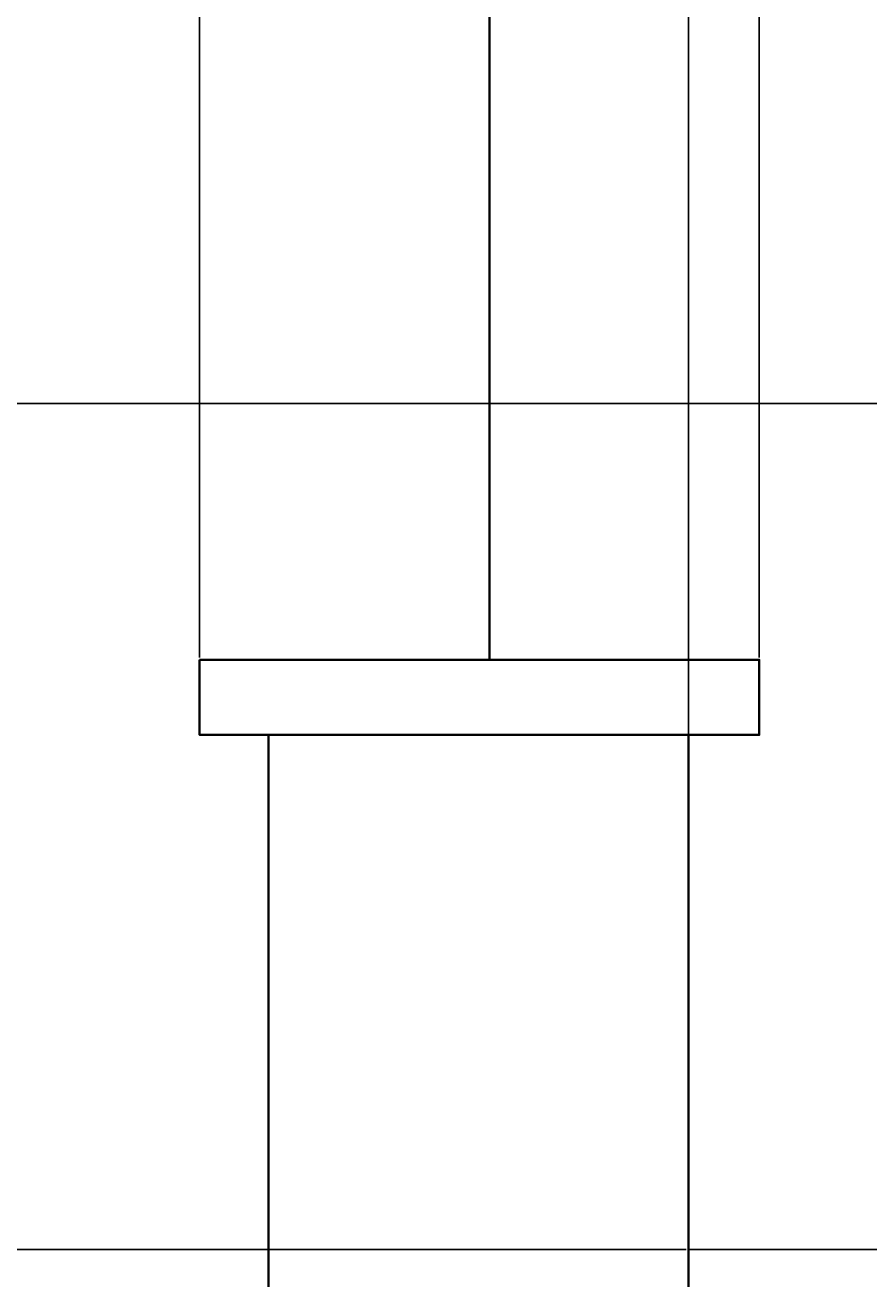
# Model space of a CAD drawing. Units: inches. Extents: x -6 to 289, y -8 to 323.
# Tile 20 of 107: x 102 to 126, y 50 to 87. Entities that reach past the tile are written whole.
import ezdxf

# ---------------------------------------------------------------- set-up
doc = ezdxf.new("R2010")
doc.units = ezdxf.units.IN
doc.header["$MEASUREMENT"] = 0
for name, color, linetype, lineweight in [('A-ANNO-DIMS', 2, 'Continuous', 18), ('A-DOOR', 3, 'Continuous', 25), ('A-ELEV', 7, 'Continuous', 35)]:
    doc.layers.add(name, color=color, linetype=linetype, lineweight=lineweight)
doc.styles.get("Standard").update_dxf_attribs({"font": 'arial.ttf'})
doc.dimstyles.get("Standard").update_dxf_attribs({"dimtxt": 0.18, "dimasz": 0.18, "dimexe": 0.18, "dimexo": 0.0625, "dimgap": 0.09, "dimtad": 0, "dimtih": 1, "dimtoh": 1, "dimdec": 4, "dimzin": 0, "dimdsep": 46, "dimtxsty": 'Standard', "dimcen": 0.09, "dimadec": 0, "dimazin": 0, "dimtfac": 1, "dimtdec": 4, "dimtofl": 0, "dimtmove": 0, "dimatfit": 3, "dimfxl": 1, "dimtolj": 1, "dimtzin": 0, "dimarcsym": 0})

# ---------------------------------------------------------------- blocks, each defined once
blk = doc.blocks.new('*D16')
at = {"layer": 'A-ANNO-DIMS', "color": 0, "lineweight": -2, "transparency": 16777216}
for p, q in [((9.943, 68.37), (9.943, -8.391)), ((272.973, 68.37), (272.973, -8.391)), ((10.123, -8.211), (140.993, -8.211)), ((272.793, -8.211), (141.923, -8.211))]:
    blk.add_line(p, q, dxfattribs=at)
at = {"layer": 'A-ANNO-DIMS', "color": 0, "transparency": 16777216}
for points in [[(10.123, -8.181), (10.123, -8.241), (9.943, -8.211)], [(272.793, -8.181), (272.793, -8.241), (272.973, -8.211)]]:
    blk.add_solid(points, dxfattribs=at)
at = {"layer": 'Defpoints', "color": 0, "transparency": 16777216}
for p in [(9.943, 68.432), (272.973, 68.432), (272.973, -8.211)]:
    blk.add_point(p, dxfattribs=at)
at = {"layer": 'A-ANNO-DIMS', "color": 0, "transparency": 16777216, "insert": (141.458, -8.211), "char_height": 0.18, "attachment_point": 5}
blk.add_mtext('\\A1;263.03', dxfattribs=at)
blk = doc.blocks.new('*D58')
at = {"layer": 'A-ANNO-DIMS', "color": 0, "lineweight": -2, "transparency": 16777216}
for p, q in [((106.634, 68.495), (106.634, 322.969)), ((106.814, 322.789), (114.479, 322.789)), ((122.914, 322.789), (115.249, 322.789)), ((123.094, 68.495), (123.094, 322.969))]:
    blk.add_line(p, q, dxfattribs=at)
at = {"layer": 'A-ANNO-DIMS', "color": 0, "transparency": 16777216}
for points in [[(106.814, 322.819), (106.814, 322.759), (106.634, 322.789)], [(122.914, 322.819), (122.914, 322.759), (123.094, 322.789)]]:
    blk.add_solid(points, dxfattribs=at)
at = {"layer": 'Defpoints', "color": 0, "transparency": 16777216}
for p in [(123.094, 322.789), (106.634, 68.432), (123.094, 68.432)]:
    blk.add_point(p, dxfattribs=at)
at = {"layer": 'A-ANNO-DIMS', "color": 0, "transparency": 16777216, "insert": (114.864, 322.789), "char_height": 0.18, "attachment_point": 5}
blk.add_mtext('\\A1;16.46', dxfattribs=at)
blk = doc.blocks.new('*D73')
at = {"layer": 'A-ANNO-DIMS', "color": 0, "lineweight": -2, "transparency": 16777216}
for p, q in [((121.008, 51.148), (121.008, 322.969)), ((121.188, 322.789), (127.697, 322.789)), ((135.116, 322.789), (128.607, 322.789)), ((135.296, 51.148), (135.296, 322.969))]:
    blk.add_line(p, q, dxfattribs=at)
at = {"layer": 'A-ANNO-DIMS', "color": 0, "transparency": 16777216}
for points in [[(121.188, 322.819), (121.188, 322.759), (121.008, 322.789)], [(135.116, 322.819), (135.116, 322.759), (135.296, 322.789)]]:
    blk.add_solid(points, dxfattribs=at)
at = {"layer": 'Defpoints', "color": 0, "transparency": 16777216}
for p in [(135.296, 322.789), (121.008, 51.085), (135.296, 51.085)]:
    blk.add_point(p, dxfattribs=at)
at = {"layer": 'A-ANNO-DIMS', "color": 0, "transparency": 16777216, "insert": (128.152, 322.789), "char_height": 0.18, "attachment_point": 5}
blk.add_mtext('\\A1;14.288', dxfattribs=at)
blk = doc.blocks.new('*D85')
at = {"layer": 'A-ANNO-DIMS', "color": 0, "lineweight": -2, "transparency": 16777216}
for p, q in [((120.945, 51.085), (-5.737, 51.085)), ((-5.557, 50.905), (-5.557, 49.767)), ((-5.557, 48.265), (-5.557, 49.403)), ((123.945, 48.085), (-5.737, 48.085))]:
    blk.add_line(p, q, dxfattribs=at)
at = {"layer": 'A-ANNO-DIMS', "color": 0, "transparency": 16777216}
for points in [[(-5.587, 50.905), (-5.527, 50.905), (-5.557, 51.085)], [(-5.587, 48.265), (-5.527, 48.265), (-5.557, 48.085)]]:
    blk.add_solid(points, dxfattribs=at)
at = {"layer": 'Defpoints', "color": 0, "transparency": 16777216}
for p in [(-5.557, 51.085), (121.008, 51.085), (124.008, 48.085)]:
    blk.add_point(p, dxfattribs=at)
at = {"layer": 'A-ANNO-DIMS', "color": 0, "transparency": 16777216, "insert": (-5.557, 49.585), "char_height": 0.18, "attachment_point": 5}
blk.add_mtext('\\A1;3', dxfattribs=at)
blk = doc.blocks.new('*D86')
at = {"layer": 'A-ANNO-DIMS', "color": 0, "lineweight": -2, "transparency": 16777216}
for p, q in [((166.233, 75.971), (-5.737, 75.971)), ((-5.557, 75.791), (-5.557, 63.71)), ((-5.557, 51.265), (-5.557, 63.346)), ((120.945, 51.085), (-5.737, 51.085))]:
    blk.add_line(p, q, dxfattribs=at)
at = {"layer": 'A-ANNO-DIMS', "color": 0, "transparency": 16777216}
for points in [[(-5.587, 75.791), (-5.527, 75.791), (-5.557, 75.971)], [(-5.587, 51.265), (-5.527, 51.265), (-5.557, 51.085)]]:
    blk.add_solid(points, dxfattribs=at)
at = {"layer": 'Defpoints', "color": 0, "transparency": 16777216}
for p in [(-5.557, 75.971), (166.296, 75.971), (121.008, 51.085)]:
    blk.add_point(p, dxfattribs=at)
at = {"layer": 'A-ANNO-DIMS', "color": 0, "transparency": 16777216, "insert": (-5.557, 63.528), "char_height": 0.18, "attachment_point": 5}
blk.add_mtext('\\A1;24.886', dxfattribs=at)
blk = doc.blocks.new('*D87')
at = {"layer": 'A-ANNO-DIMS', "color": 0, "lineweight": -2, "transparency": 16777216}
for p, q in [((142.233, 108.948), (-5.737, 108.948)), ((-5.557, 108.768), (-5.557, 92.641)), ((-5.557, 76.151), (-5.557, 92.277)), ((166.233, 75.971), (-5.737, 75.971))]:
    blk.add_line(p, q, dxfattribs=at)
at = {"layer": 'A-ANNO-DIMS', "color": 0, "transparency": 16777216}
for points in [[(-5.587, 108.768), (-5.527, 108.768), (-5.557, 108.948)], [(-5.587, 76.151), (-5.527, 76.151), (-5.557, 75.971)]]:
    blk.add_solid(points, dxfattribs=at)
at = {"layer": 'Defpoints', "color": 0, "transparency": 16777216}
for p in [(-5.557, 108.948), (142.296, 108.948), (166.296, 75.971)]:
    blk.add_point(p, dxfattribs=at)
at = {"layer": 'A-ANNO-DIMS', "color": 0, "transparency": 16777216, "insert": (-5.557, 92.459), "char_height": 0.18, "attachment_point": 5}
blk.add_mtext('\\A1;32.98', dxfattribs=at)

msp = doc.modelspace()

# ---------------------------------------------------------------- linework, layer by layer
at = {"layer": 'A-DOOR'}
msp.add_lwpolyline([(121.008, 51.0851), (247.2408, 51.0851), (247.2408, 7.2888), (121.008, 7.2888)], close=True, dxfattribs=at)
at = {"layer": 'A-ELEV'}
msp.add_line((115.1638, 127.2888), (115.1638, 68.4322), dxfattribs=at)
msp.add_lwpolyline([(106.634, 68.4322), (123.094, 68.4322), (123.094, 66.2238), (106.634, 66.2238)], close=True, dxfattribs=at)
for points in [[(121.008, 68.4322), (108.6602, 68.4322)], [(108.6602, 66.2238), (108.6602, 7.2888), (121.008, 7.2888), (121.008, 66.2238)]]:
    msp.add_lwpolyline(points, dxfattribs=at)

# ---------------------------------------------------------------- dimensions: what is measured, and where the dimension line sits
at = {"layer": 'A-ANNO-DIMS'}
for base, p1, p2, override, picture, middle in [((123.094, 322.7888), (106.634, 68.4322), (123.094, 68.4322), {"dimdec": 2, "dimlfac": 1, "dimrnd": 0, "dimzin": 0, "dimdsep": 46, "dimlunit": 2}, '*D58', (114.864, 322.7888)), ((135.296, 322.7888), (121.008, 51.0851), (135.296, 51.0851), {"dimdec": 3, "dimlfac": 1, "dimrnd": 0, "dimzin": 0, "dimdsep": 46, "dimlunit": 2}, '*D73', (128.152, 322.7888)), ((272.9733, -8.2112), (9.943, 68.4322), (272.9733, 68.4322), {"dimdec": 2, "dimlfac": 1, "dimrnd": 0, "dimzin": 0, "dimdsep": 46, "dimlunit": 2}, '*D16', (141.4581, -8.2112))]:
    dim = msp.add_linear_dim(base=base, p1=p1, p2=p2, dimstyle='Standard', override=override, dxfattribs=at)
    dim.commit()
    dim.dimension.update_dxf_attribs({"geometry": picture, "text_midpoint": middle})
for base, p1, p2, override, picture, middle in [((-5.557, 108.9477), (166.296, 75.9706), (142.296, 108.9477), {"dimdec": 2, "dimlfac": 1, "dimrnd": 0, "dimzin": 0, "dimdsep": 46, "dimlunit": 2}, '*D87', (-5.557, 92.4592)), ((-5.557, 75.97064), (121.00798, 51.08513), (166.29599, 75.97064), {"dimdec": 3, "dimlfac": 1, "dimrnd": 0, "dimzin": 0, "dimdsep": 46, "dimlunit": 2}, '*D86', (-5.557, 63.52788)), ((-5.557, 51.0851), (124.008, 48.0851), (121.008, 51.0851), {"dimdec": 0, "dimlfac": 1, "dimrnd": 0, "dimzin": 0, "dimdsep": 46, "dimlunit": 2}, '*D85', (-5.557, 49.5851))]:
    dim = msp.add_linear_dim(base=base, p1=p1, p2=p2, angle=90, dimstyle='Standard', override=override, dxfattribs=at)
    dim.commit()
    dim.dimension.update_dxf_attribs({"geometry": picture, "text_midpoint": middle})

doc.saveas('drawing.dxf')
